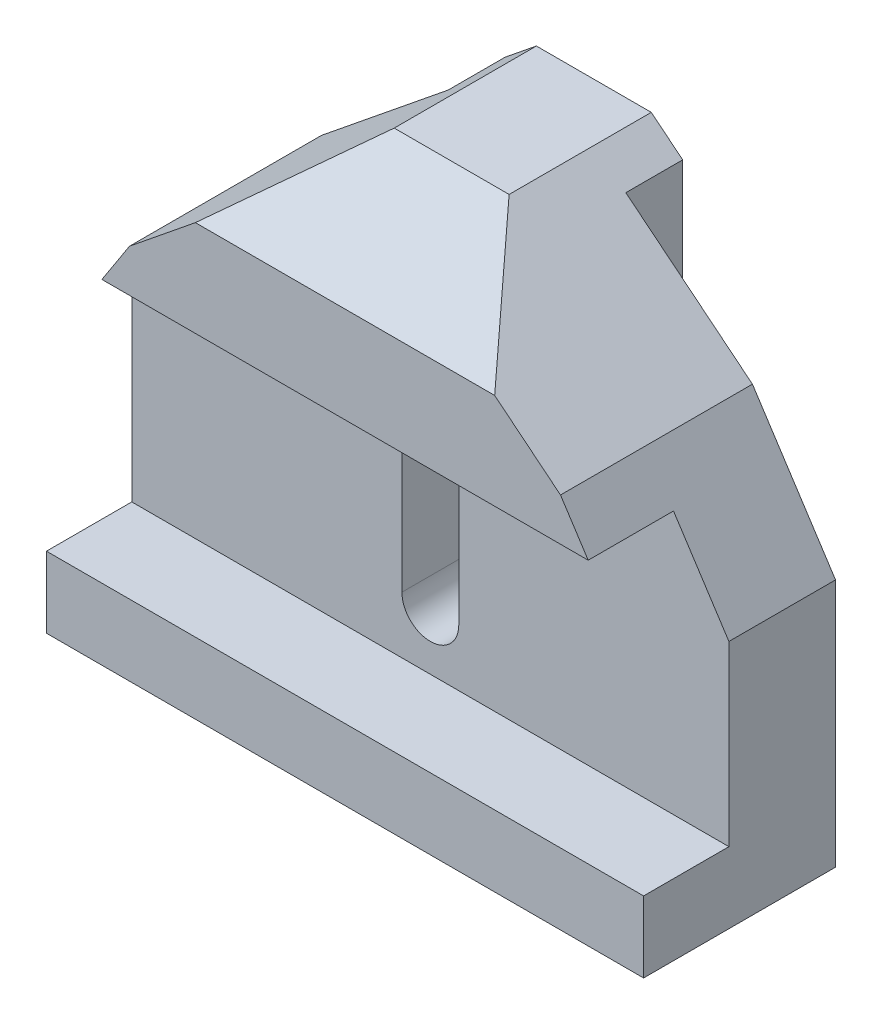
ISO-10303-21;
HEADER;
FILE_DESCRIPTION(('STEP AP214'),'2;1');
FILE_NAME('part.step','',(''),(''),'','','');
FILE_SCHEMA(('AUTOMOTIVE_DESIGN { 1 0 10303 214 1 1 1 1 }'));
ENDSEC;
DATA;
#1=APPLICATION_CONTEXT('core data for automotive mechanical design processes');
#2=APPLICATION_PROTOCOL_DEFINITION('international standard','automotive_design',2000,#1);
#3=PRODUCT_CONTEXT('',#1,'mechanical');
#4=PRODUCT('Part','Part','',(#3));
#5=PRODUCT_RELATED_PRODUCT_CATEGORY('part','',(#4));
#6=PRODUCT_DEFINITION_FORMATION('','',#4);
#7=PRODUCT_DEFINITION_CONTEXT('part definition',#1,'design');
#8=PRODUCT_DEFINITION('design','',#6,#7);
#9=PRODUCT_DEFINITION_SHAPE('','',#8);
#10=(LENGTH_UNIT() NAMED_UNIT(*) SI_UNIT(.MILLI.,.METRE.));
#11=(NAMED_UNIT(*) PLANE_ANGLE_UNIT() SI_UNIT($,.RADIAN.));
#12=(NAMED_UNIT(*) SI_UNIT($,.STERADIAN.) SOLID_ANGLE_UNIT());
#13=UNCERTAINTY_MEASURE_WITH_UNIT(LENGTH_MEASURE(1.E-05),#10,'distance_accuracy_value','');
#14=(GEOMETRIC_REPRESENTATION_CONTEXT(3) GLOBAL_UNCERTAINTY_ASSIGNED_CONTEXT((#13)) GLOBAL_UNIT_ASSIGNED_CONTEXT((#10,
#11,#12)) REPRESENTATION_CONTEXT('',''));
#15=CARTESIAN_POINT('',(0.,0.,0.));
#16=DIRECTION('',(0.,0.,1.));
#17=DIRECTION('',(1.,0.,0.));
#18=AXIS2_PLACEMENT_3D('',#15,#16,#17);
#19=CARTESIAN_POINT('',(-84.,0.,23.));
#20=DIRECTION('',(0.,0.,1.));
#21=DIRECTION('',(0.,-1.,0.));
#22=AXIS2_PLACEMENT_3D('',#19,#20,#21);
#23=PLANE('',#22);
#24=CARTESIAN_POINT('',(-42.,18.,23.));
#25=DIRECTION('',(0.,0.,1.));
#26=DIRECTION('',(1.,0.,0.));
#27=AXIS2_PLACEMENT_3D('',#24,#25,#26);
#28=CIRCLE('',#27,4.);
#29=CARTESIAN_POINT('',(-46.,18.,23.));
#30=VERTEX_POINT('',#29);
#31=CARTESIAN_POINT('',(-38.,18.,23.));
#32=VERTEX_POINT('',#31);
#33=EDGE_CURVE('E54',#30,#32,#28,.T.);
#34=ORIENTED_EDGE('',*,*,#33,.F.);
#35=DIRECTION('',(0.,1.,0.));
#36=VECTOR('',#35,1.);
#37=CARTESIAN_POINT('',(-46.,18.,23.));
#38=LINE('',#37,#36);
#39=CARTESIAN_POINT('',(-46.,39.,23.));
#40=VERTEX_POINT('',#39);
#41=EDGE_CURVE('E199',#30,#40,#38,.T.);
#42=ORIENTED_EDGE('',*,*,#41,.T.);
#43=CARTESIAN_POINT('',(-42.,39.,23.));
#44=DIRECTION('',(0.,0.,1.));
#45=DIRECTION('',(1.,0.,0.));
#46=AXIS2_PLACEMENT_3D('',#43,#44,#45);
#47=CIRCLE('',#46,4.);
#48=CARTESIAN_POINT('',(-38.,39.,23.));
#49=VERTEX_POINT('',#48);
#50=EDGE_CURVE('E184',#49,#40,#47,.T.);
#51=ORIENTED_EDGE('',*,*,#50,.F.);
#52=DIRECTION('',(0.,1.,0.));
#53=VECTOR('',#52,1.);
#54=CARTESIAN_POINT('',(-38.,18.,23.));
#55=LINE('',#54,#53);
#56=EDGE_CURVE('E191',#32,#49,#55,.T.);
#57=ORIENTED_EDGE('',*,*,#56,.F.);
#58=EDGE_LOOP('',(#34,#42,#51,#57));
#59=FACE_BOUND('',#58,.T.);
#60=DIRECTION('',(0.544639035015022,-0.838670567945427,0.));
#61=VECTOR('',#60,1.);
#62=CARTESIAN_POINT('',(-8.93001548207051,48.7510179671623,23.));
#63=LINE('',#62,#61);
#64=CARTESIAN_POINT('',(-7.79289111837003,47.,23.));
#65=VERTEX_POINT('',#64);
#66=CARTESIAN_POINT('',(0.,35.,23.));
#67=VERTEX_POINT('',#66);
#68=EDGE_CURVE('E262',#65,#67,#63,.T.);
#69=ORIENTED_EDGE('',*,*,#68,.F.);
#70=DIRECTION('',(1.,0.,0.));
#71=VECTOR('',#70,1.);
#72=CARTESIAN_POINT('',(-84.,47.,23.));
#73=LINE('',#72,#71);
#74=CARTESIAN_POINT('',(-76.20710888163,47.,23.));
#75=VERTEX_POINT('',#74);
#76=EDGE_CURVE('E295',#75,#65,#73,.T.);
#77=ORIENTED_EDGE('',*,*,#76,.F.);
#78=DIRECTION('',(0.544639035015022,0.838670567945427,0.));
#79=VECTOR('',#78,1.);
#80=CARTESIAN_POINT('',(-99.9870455087454,10.3821087461733,23.));
#81=LINE('',#80,#79);
#82=CARTESIAN_POINT('',(-84.,35.,23.));
#83=VERTEX_POINT('',#82);
#84=EDGE_CURVE('E267',#83,#75,#81,.T.);
#85=ORIENTED_EDGE('',*,*,#84,.F.);
#86=DIRECTION('',(0.,-1.,0.));
#87=VECTOR('',#86,1.);
#88=CARTESIAN_POINT('',(-84.,0.,23.));
#89=LINE('',#88,#87);
#90=CARTESIAN_POINT('',(-84.,10.,23.));
#91=VERTEX_POINT('',#90);
#92=EDGE_CURVE('E273',#83,#91,#89,.T.);
#93=ORIENTED_EDGE('',*,*,#92,.T.);
#94=DIRECTION('',(1.,0.,0.));
#95=VECTOR('',#94,1.);
#96=CARTESIAN_POINT('',(-84.,10.,23.));
#97=LINE('',#96,#95);
#98=CARTESIAN_POINT('',(0.,10.,23.));
#99=VERTEX_POINT('',#98);
#100=EDGE_CURVE('E284',#91,#99,#97,.T.);
#101=ORIENTED_EDGE('',*,*,#100,.T.);
#102=DIRECTION('',(0.,-1.,0.));
#103=VECTOR('',#102,1.);
#104=CARTESIAN_POINT('',(0.,0.,23.));
#105=LINE('',#104,#103);
#106=EDGE_CURVE('E274',#67,#99,#105,.T.);
#107=ORIENTED_EDGE('',*,*,#106,.F.);
#108=EDGE_LOOP('',(#69,#77,#85,#93,#101,#107));
#109=FACE_BOUND('',#108,.T.);
#110=ADVANCED_FACE('F41',(#59,#109),#23,.T.);
#111=CARTESIAN_POINT('',(-84.,47.,0.));
#112=DIRECTION('',(0.,-1.,0.));
#113=DIRECTION('',(0.,0.,-1.));
#114=AXIS2_PLACEMENT_3D('',#111,#112,#113);
#115=PLANE('',#114);
#116=DIRECTION('',(0.,0.,-1.));
#117=VECTOR('',#116,1.);
#118=CARTESIAN_POINT('',(-7.79289111837002,47.,0.));
#119=LINE('',#118,#117);
#120=CARTESIAN_POINT('',(-7.79289111837003,47.,35.));
#121=VERTEX_POINT('',#120);
#122=EDGE_CURVE('E254',#121,#65,#119,.T.);
#123=ORIENTED_EDGE('',*,*,#122,.F.);
#124=DIRECTION('',(1.,0.,0.));
#125=VECTOR('',#124,1.);
#126=CARTESIAN_POINT('',(-84.,47.,35.));
#127=LINE('',#126,#125);
#128=CARTESIAN_POINT('',(-76.20710888163,47.,35.));
#129=VERTEX_POINT('',#128);
#130=EDGE_CURVE('E296',#129,#121,#127,.T.);
#131=ORIENTED_EDGE('',*,*,#130,.F.);
#132=DIRECTION('',(0.,0.,1.));
#133=VECTOR('',#132,1.);
#134=CARTESIAN_POINT('',(-76.20710888163,47.,0.));
#135=LINE('',#134,#133);
#136=EDGE_CURVE('E268',#75,#129,#135,.T.);
#137=ORIENTED_EDGE('',*,*,#136,.F.);
#138=ORIENTED_EDGE('',*,*,#76,.T.);
#139=EDGE_LOOP('',(#123,#131,#137,#138));
#140=FACE_BOUND('',#139,.T.);
#141=ADVANCED_FACE('F368',(#140),#115,.T.);
#142=CARTESIAN_POINT('',(-84.,0.,35.));
#143=DIRECTION('',(0.,0.,1.));
#144=DIRECTION('',(1.,0.,0.));
#145=AXIS2_PLACEMENT_3D('',#142,#143,#144);
#146=PLANE('',#145);
#147=DIRECTION('',(0.544639035015022,-0.838670567945427,0.));
#148=VECTOR('',#147,1.);
#149=CARTESIAN_POINT('',(0.,35.,35.));
#150=LINE('',#149,#148);
#151=CARTESIAN_POINT('',(-11.689336677555,53.,35.));
#152=VERTEX_POINT('',#151);
#153=EDGE_CURVE('E250',#152,#121,#150,.T.);
#154=ORIENTED_EDGE('',*,*,#153,.F.);
#155=DIRECTION('',(0.777145961456972,-0.629320391049836,0.));
#156=VECTOR('',#155,1.);
#157=CARTESIAN_POINT('',(-11.689336677555,53.,35.));
#158=LINE('',#157,#156);
#159=CARTESIAN_POINT('',(-20.9472210263923,60.4968869268543,35.));
#160=VERTEX_POINT('',#159);
#161=EDGE_CURVE('E242',#160,#152,#158,.T.);
#162=ORIENTED_EDGE('',*,*,#161,.F.);
#163=DIRECTION('',(1.,0.,0.));
#164=VECTOR('',#163,1.);
#165=CARTESIAN_POINT('',(-84.,60.4968869268543,35.));
#166=LINE('',#165,#164);
#167=CARTESIAN_POINT('',(-63.0527789736078,60.4968869268543,35.));
#168=VERTEX_POINT('',#167);
#169=EDGE_CURVE('E301',#168,#160,#166,.T.);
#170=ORIENTED_EDGE('',*,*,#169,.F.);
#171=DIRECTION('',(0.777145961456972,0.629320391049836,0.));
#172=VECTOR('',#171,1.);
#173=CARTESIAN_POINT('',(-72.310663322445,53.,35.));
#174=LINE('',#173,#172);
#175=CARTESIAN_POINT('',(-72.310663322445,53.,35.));
#176=VERTEX_POINT('',#175);
#177=EDGE_CURVE('E260',#176,#168,#174,.T.);
#178=ORIENTED_EDGE('',*,*,#177,.F.);
#179=DIRECTION('',(0.544639035015022,0.838670567945427,0.));
#180=VECTOR('',#179,1.);
#181=CARTESIAN_POINT('',(-84.,35.,35.));
#182=LINE('',#181,#180);
#183=EDGE_CURVE('E247',#129,#176,#182,.T.);
#184=ORIENTED_EDGE('',*,*,#183,.F.);
#185=ORIENTED_EDGE('',*,*,#130,.T.);
#186=EDGE_LOOP('',(#154,#162,#170,#178,#184,#185));
#187=FACE_BOUND('',#186,.T.);
#188=ADVANCED_FACE('F375',(#187),#146,.T.);
#189=CARTESIAN_POINT('',(-84.,57.0386412959202,39.9388866046431));
#190=DIRECTION('',(0.,0.819152044288991,0.573576436351047));
#191=DIRECTION('',(0.,-0.573576436351047,0.819152044288991));
#192=AXIS2_PLACEMENT_3D('',#189,#190,#191);
#193=PLANE('',#192);
#194=DIRECTION('',(0.578003525978811,-0.468058026468054,0.668456137539998));
#195=VECTOR('',#194,1.);
#196=CARTESIAN_POINT('',(-39.1685740328013,75.2522476546541,13.9271609878319));
#197=LINE('',#196,#195);
#198=CARTESIAN_POINT('',(-33.9174854951861,71.,20.));
#199=VERTEX_POINT('',#198);
#200=EDGE_CURVE('E275',#199,#160,#197,.T.);
#201=ORIENTED_EDGE('',*,*,#200,.F.);
#202=DIRECTION('',(1.,0.,0.));
#203=VECTOR('',#202,1.);
#204=CARTESIAN_POINT('',(-84.,71.,20.));
#205=LINE('',#204,#203);
#206=CARTESIAN_POINT('',(-50.082514504814,71.,20.));
#207=VERTEX_POINT('',#206);
#208=EDGE_CURVE('E302',#207,#199,#205,.T.);
#209=ORIENTED_EDGE('',*,*,#208,.F.);
#210=DIRECTION('',(0.578003525978811,0.468058026468054,-0.668456137539998));
#211=VECTOR('',#210,1.);
#212=CARTESIAN_POINT('',(-72.8948243548895,52.5269557231117,46.3822413624967));
#213=LINE('',#212,#211);
#214=EDGE_CURVE('E266',#168,#207,#213,.T.);
#215=ORIENTED_EDGE('',*,*,#214,.F.);
#216=ORIENTED_EDGE('',*,*,#169,.T.);
#217=EDGE_LOOP('',(#201,#209,#215,#216));
#218=FACE_BOUND('',#217,.T.);
#219=ADVANCED_FACE('F378',(#218),#193,.T.);
#220=CARTESIAN_POINT('',(-84.,71.,0.));
#221=DIRECTION('',(0.,1.,0.));
#222=DIRECTION('',(0.,0.,1.));
#223=AXIS2_PLACEMENT_3D('',#220,#221,#222);
#224=PLANE('',#223);
#225=DIRECTION('',(0.,0.,1.));
#226=VECTOR('',#225,1.);
#227=CARTESIAN_POINT('',(-33.9174854951861,71.,-49.));
#228=LINE('',#227,#226);
#229=CARTESIAN_POINT('',(-33.9174854951861,71.,0.));
#230=VERTEX_POINT('',#229);
#231=EDGE_CURVE('E249',#230,#199,#228,.T.);
#232=ORIENTED_EDGE('',*,*,#231,.F.);
#233=DIRECTION('',(1.,0.,0.));
#234=VECTOR('',#233,1.);
#235=CARTESIAN_POINT('',(-84.,71.,0.));
#236=LINE('',#235,#234);
#237=CARTESIAN_POINT('',(-50.082514504814,71.,0.));
#238=VERTEX_POINT('',#237);
#239=EDGE_CURVE('E310',#238,#230,#236,.T.);
#240=ORIENTED_EDGE('',*,*,#239,.F.);
#241=DIRECTION('',(0.,0.,1.));
#242=VECTOR('',#241,1.);
#243=CARTESIAN_POINT('',(-50.082514504814,71.,-49.));
#244=LINE('',#243,#242);
#245=EDGE_CURVE('E243',#238,#207,#244,.T.);
#246=ORIENTED_EDGE('',*,*,#245,.T.);
#247=ORIENTED_EDGE('',*,*,#208,.T.);
#248=EDGE_LOOP('',(#232,#240,#246,#247));
#249=FACE_BOUND('',#248,.T.);
#250=ADVANCED_FACE('F386',(#249),#224,.T.);
#251=CARTESIAN_POINT('',(-84.,0.,0.));
#252=DIRECTION('',(0.,0.,-1.));
#253=DIRECTION('',(-1.,0.,0.));
#254=AXIS2_PLACEMENT_3D('',#251,#252,#253);
#255=PLANE('',#254);
#256=CARTESIAN_POINT('',(-42.,18.,0.));
#257=DIRECTION('',(0.,0.,-1.));
#258=DIRECTION('',(-1.,0.,0.));
#259=AXIS2_PLACEMENT_3D('',#256,#257,#258);
#260=CIRCLE('',#259,4.);
#261=CARTESIAN_POINT('',(-38.,18.,0.));
#262=VERTEX_POINT('',#261);
#263=CARTESIAN_POINT('',(-46.,18.,0.));
#264=VERTEX_POINT('',#263);
#265=EDGE_CURVE('E11',#262,#264,#260,.T.);
#266=ORIENTED_EDGE('',*,*,#265,.F.);
#267=DIRECTION('',(0.,-1.,0.));
#268=VECTOR('',#267,1.);
#269=CARTESIAN_POINT('',(-38.,0.,0.));
#270=LINE('',#269,#268);
#271=CARTESIAN_POINT('',(-38.,39.,0.));
#272=VERTEX_POINT('',#271);
#273=EDGE_CURVE('E345',#272,#262,#270,.T.);
#274=ORIENTED_EDGE('',*,*,#273,.F.);
#275=CARTESIAN_POINT('',(-42.,39.,0.));
#276=DIRECTION('',(0.,0.,-1.));
#277=DIRECTION('',(-1.,0.,0.));
#278=AXIS2_PLACEMENT_3D('',#275,#276,#277);
#279=CIRCLE('',#278,4.);
#280=CARTESIAN_POINT('',(-46.,39.,0.));
#281=VERTEX_POINT('',#280);
#282=EDGE_CURVE('E189',#281,#272,#279,.T.);
#283=ORIENTED_EDGE('',*,*,#282,.F.);
#284=DIRECTION('',(0.,-1.,0.));
#285=VECTOR('',#284,1.);
#286=CARTESIAN_POINT('',(-46.,0.,0.));
#287=LINE('',#286,#285);
#288=EDGE_CURVE('E48',#281,#264,#287,.T.);
#289=ORIENTED_EDGE('',*,*,#288,.T.);
#290=EDGE_LOOP('',(#266,#274,#283,#289));
#291=FACE_BOUND('',#290,.T.);
#292=DIRECTION('',(0.,1.,0.));
#293=VECTOR('',#292,1.);
#294=CARTESIAN_POINT('',(-54.5,-33.,0.));
#295=LINE('',#294,#293);
#296=CARTESIAN_POINT('',(-54.5,0.,0.));
#297=VERTEX_POINT('',#296);
#298=CARTESIAN_POINT('',(-54.5,67.4227907791278,0.));
#299=VERTEX_POINT('',#298);
#300=EDGE_CURVE('E208',#297,#299,#295,.T.);
#301=ORIENTED_EDGE('',*,*,#300,.T.);
#302=DIRECTION('',(-0.777145961456972,-0.629320391049836,0.));
#303=VECTOR('',#302,1.);
#304=CARTESIAN_POINT('',(-105.291417957253,26.2927114940107,0.));
#305=LINE('',#304,#303);
#306=EDGE_CURVE('E323',#238,#299,#305,.T.);
#307=ORIENTED_EDGE('',*,*,#306,.F.);
#308=ORIENTED_EDGE('',*,*,#239,.T.);
#309=DIRECTION('',(-0.777145961456972,0.629320391049836,0.));
#310=VECTOR('',#309,1.);
#311=CARTESIAN_POINT('',(-29.4408730570935,67.3749107248305,0.));
#312=LINE('',#311,#310);
#313=CARTESIAN_POINT('',(-29.5,67.4227907791278,0.));
#314=VERTEX_POINT('',#313);
#315=EDGE_CURVE('E328',#314,#230,#312,.T.);
#316=ORIENTED_EDGE('',*,*,#315,.F.);
#317=DIRECTION('',(0.,1.,0.));
#318=VECTOR('',#317,1.);
#319=CARTESIAN_POINT('',(-29.5,-33.,0.));
#320=LINE('',#319,#318);
#321=CARTESIAN_POINT('',(-29.5,0.,0.));
#322=VERTEX_POINT('',#321);
#323=EDGE_CURVE('E217',#322,#314,#320,.T.);
#324=ORIENTED_EDGE('',*,*,#323,.F.);
#325=DIRECTION('',(1.,0.,0.));
#326=VECTOR('',#325,1.);
#327=CARTESIAN_POINT('',(-84.,0.,0.));
#328=LINE('',#327,#326);
#329=EDGE_CURVE('E309',#297,#322,#328,.T.);
#330=ORIENTED_EDGE('',*,*,#329,.F.);
#331=EDGE_LOOP('',(#301,#307,#308,#316,#324,#330));
#332=FACE_BOUND('',#331,.T.);
#333=ADVANCED_FACE('F350',(#291,#332),#255,.T.);
#334=CARTESIAN_POINT('',(-84.,0.,0.));
#335=DIRECTION('',(0.,1.,0.));
#336=DIRECTION('',(0.,0.,1.));
#337=AXIS2_PLACEMENT_3D('',#334,#335,#336);
#338=PLANE('',#337);
#339=DIRECTION('',(1.,0.,0.));
#340=VECTOR('',#339,1.);
#341=CARTESIAN_POINT('',(-84.,0.,8.));
#342=LINE('',#341,#340);
#343=CARTESIAN_POINT('',(-84.,0.,8.));
#344=VERTEX_POINT('',#343);
#345=CARTESIAN_POINT('',(-54.5,0.,8.));
#346=VERTEX_POINT('',#345);
#347=EDGE_CURVE('E226',#344,#346,#342,.T.);
#348=ORIENTED_EDGE('',*,*,#347,.T.);
#349=DIRECTION('',(0.,0.,-1.));
#350=VECTOR('',#349,1.);
#351=CARTESIAN_POINT('',(-54.5,0.,0.));
#352=LINE('',#351,#350);
#353=EDGE_CURVE('E233',#346,#297,#352,.T.);
#354=ORIENTED_EDGE('',*,*,#353,.T.);
#355=ORIENTED_EDGE('',*,*,#329,.T.);
#356=DIRECTION('',(0.,0.,1.));
#357=VECTOR('',#356,1.);
#358=CARTESIAN_POINT('',(-29.5,0.,0.));
#359=LINE('',#358,#357);
#360=CARTESIAN_POINT('',(-29.5,0.,7.99999999999999));
#361=VERTEX_POINT('',#360);
#362=EDGE_CURVE('E234',#322,#361,#359,.T.);
#363=ORIENTED_EDGE('',*,*,#362,.T.);
#364=DIRECTION('',(1.,0.,0.));
#365=VECTOR('',#364,1.);
#366=CARTESIAN_POINT('',(-84.,0.,7.99999999999998));
#367=LINE('',#366,#365);
#368=CARTESIAN_POINT('',(0.,0.,7.99999999999999));
#369=VERTEX_POINT('',#368);
#370=EDGE_CURVE('E239',#361,#369,#367,.T.);
#371=ORIENTED_EDGE('',*,*,#370,.T.);
#372=DIRECTION('',(0.,0.,1.));
#373=VECTOR('',#372,1.);
#374=CARTESIAN_POINT('',(0.,0.,0.));
#375=LINE('',#374,#373);
#376=CARTESIAN_POINT('',(0.,0.,35.));
#377=VERTEX_POINT('',#376);
#378=EDGE_CURVE('E279',#369,#377,#375,.T.);
#379=ORIENTED_EDGE('',*,*,#378,.T.);
#380=DIRECTION('',(1.,0.,0.));
#381=VECTOR('',#380,1.);
#382=CARTESIAN_POINT('',(-84.,0.,35.));
#383=LINE('',#382,#381);
#384=CARTESIAN_POINT('',(-84.,0.,35.));
#385=VERTEX_POINT('',#384);
#386=EDGE_CURVE('E312',#385,#377,#383,.T.);
#387=ORIENTED_EDGE('',*,*,#386,.F.);
#388=DIRECTION('',(0.,0.,1.));
#389=VECTOR('',#388,1.);
#390=CARTESIAN_POINT('',(-84.,0.,0.));
#391=LINE('',#390,#389);
#392=EDGE_CURVE('E283',#344,#385,#391,.T.);
#393=ORIENTED_EDGE('',*,*,#392,.F.);
#394=EDGE_LOOP('',(#348,#354,#355,#363,#371,#379,#387,#393));
#395=FACE_BOUND('',#394,.T.);
#396=ADVANCED_FACE('F394',(#395),#338,.F.);
#397=CARTESIAN_POINT('',(-84.,0.,35.));
#398=DIRECTION('',(0.,0.,-1.));
#399=DIRECTION('',(-1.,0.,0.));
#400=AXIS2_PLACEMENT_3D('',#397,#398,#399);
#401=PLANE('',#400);
#402=DIRECTION('',(0.,1.,0.));
#403=VECTOR('',#402,1.);
#404=CARTESIAN_POINT('',(0.,0.,35.));
#405=LINE('',#404,#403);
#406=CARTESIAN_POINT('',(0.,10.,35.));
#407=VERTEX_POINT('',#406);
#408=EDGE_CURVE('E286',#377,#407,#405,.T.);
#409=ORIENTED_EDGE('',*,*,#408,.T.);
#410=DIRECTION('',(1.,0.,0.));
#411=VECTOR('',#410,1.);
#412=CARTESIAN_POINT('',(-84.,10.,35.));
#413=LINE('',#412,#411);
#414=CARTESIAN_POINT('',(-84.,10.,35.));
#415=VERTEX_POINT('',#414);
#416=EDGE_CURVE('E317',#415,#407,#413,.T.);
#417=ORIENTED_EDGE('',*,*,#416,.F.);
#418=DIRECTION('',(0.,1.,0.));
#419=VECTOR('',#418,1.);
#420=CARTESIAN_POINT('',(-84.,0.,35.));
#421=LINE('',#420,#419);
#422=EDGE_CURVE('E281',#385,#415,#421,.T.);
#423=ORIENTED_EDGE('',*,*,#422,.F.);
#424=ORIENTED_EDGE('',*,*,#386,.T.);
#425=EDGE_LOOP('',(#409,#417,#423,#424));
#426=FACE_BOUND('',#425,.T.);
#427=ADVANCED_FACE('F397',(#426),#401,.F.);
#428=CARTESIAN_POINT('',(-84.,10.,0.));
#429=DIRECTION('',(0.,1.,0.));
#430=DIRECTION('',(0.,0.,1.));
#431=AXIS2_PLACEMENT_3D('',#428,#429,#430);
#432=PLANE('',#431);
#433=DIRECTION('',(0.,0.,1.));
#434=VECTOR('',#433,1.);
#435=CARTESIAN_POINT('',(0.,10.,0.));
#436=LINE('',#435,#434);
#437=EDGE_CURVE('E289',#99,#407,#436,.T.);
#438=ORIENTED_EDGE('',*,*,#437,.F.);
#439=ORIENTED_EDGE('',*,*,#100,.F.);
#440=DIRECTION('',(0.,0.,1.));
#441=VECTOR('',#440,1.);
#442=CARTESIAN_POINT('',(-84.,10.,0.));
#443=LINE('',#442,#441);
#444=EDGE_CURVE('E280',#91,#415,#443,.T.);
#445=ORIENTED_EDGE('',*,*,#444,.T.);
#446=ORIENTED_EDGE('',*,*,#416,.T.);
#447=EDGE_LOOP('',(#438,#439,#445,#446));
#448=FACE_BOUND('',#447,.T.);
#449=ADVANCED_FACE('F402',(#448),#432,.T.);
#450=CARTESIAN_POINT('',(-84.,0.,0.));
#451=DIRECTION('',(1.,0.,0.));
#452=DIRECTION('',(0.,0.,-1.));
#453=AXIS2_PLACEMENT_3D('',#450,#451,#452);
#454=PLANE('',#453);
#455=DIRECTION('',(0.,0.,-1.));
#456=VECTOR('',#455,1.);
#457=CARTESIAN_POINT('',(-84.,35.,0.));
#458=LINE('',#457,#456);
#459=CARTESIAN_POINT('',(-84.,35.,8.00000000000001));
#460=VERTEX_POINT('',#459);
#461=EDGE_CURVE('E325',#83,#460,#458,.T.);
#462=ORIENTED_EDGE('',*,*,#461,.T.);
#463=DIRECTION('',(0.,1.,0.));
#464=VECTOR('',#463,1.);
#465=CARTESIAN_POINT('',(-84.,-33.,8.));
#466=LINE('',#465,#464);
#467=EDGE_CURVE('E220',#344,#460,#466,.T.);
#468=ORIENTED_EDGE('',*,*,#467,.F.);
#469=ORIENTED_EDGE('',*,*,#392,.T.);
#470=ORIENTED_EDGE('',*,*,#422,.T.);
#471=ORIENTED_EDGE('',*,*,#444,.F.);
#472=ORIENTED_EDGE('',*,*,#92,.F.);
#473=EDGE_LOOP('',(#462,#468,#469,#470,#471,#472));
#474=FACE_BOUND('',#473,.T.);
#475=ADVANCED_FACE('F401',(#474),#454,.F.);
#476=CARTESIAN_POINT('',(0.,0.,0.));
#477=DIRECTION('',(1.,0.,0.));
#478=DIRECTION('',(0.,0.,-1.));
#479=AXIS2_PLACEMENT_3D('',#476,#477,#478);
#480=PLANE('',#479);
#481=DIRECTION('',(0.,1.,0.));
#482=VECTOR('',#481,1.);
#483=CARTESIAN_POINT('',(0.,-33.,7.99999999999999));
#484=LINE('',#483,#482);
#485=CARTESIAN_POINT('',(0.,35.,7.99999999999999));
#486=VERTEX_POINT('',#485);
#487=EDGE_CURVE('E210',#369,#486,#484,.T.);
#488=ORIENTED_EDGE('',*,*,#487,.T.);
#489=DIRECTION('',(0.,0.,-1.));
#490=VECTOR('',#489,1.);
#491=CARTESIAN_POINT('',(0.,35.,0.));
#492=LINE('',#491,#490);
#493=EDGE_CURVE('E300',#67,#486,#492,.T.);
#494=ORIENTED_EDGE('',*,*,#493,.F.);
#495=ORIENTED_EDGE('',*,*,#106,.T.);
#496=ORIENTED_EDGE('',*,*,#437,.T.);
#497=ORIENTED_EDGE('',*,*,#408,.F.);
#498=ORIENTED_EDGE('',*,*,#378,.F.);
#499=EDGE_LOOP('',(#488,#494,#495,#496,#497,#498));
#500=FACE_BOUND('',#499,.T.);
#501=ADVANCED_FACE('F381',(#500),#480,.T.);
#502=CARTESIAN_POINT('',(0.,35.,-49.));
#503=DIRECTION('',(-0.838670567945427,-0.544639035015022,0.));
#504=DIRECTION('',(0.544639035015022,-0.838670567945427,0.));
#505=AXIS2_PLACEMENT_3D('',#502,#503,#504);
#506=PLANE('',#505);
#507=ORIENTED_EDGE('',*,*,#493,.T.);
#508=DIRECTION('',(-0.544639035015022,0.838670567945427,0.));
#509=VECTOR('',#508,1.);
#510=CARTESIAN_POINT('',(0.,35.,7.99999999999999));
#511=LINE('',#510,#509);
#512=CARTESIAN_POINT('',(-11.689336677555,53.,7.99999999999999));
#513=VERTEX_POINT('',#512);
#514=EDGE_CURVE('E240',#486,#513,#511,.T.);
#515=ORIENTED_EDGE('',*,*,#514,.T.);
#516=DIRECTION('',(0.,0.,1.));
#517=VECTOR('',#516,1.);
#518=CARTESIAN_POINT('',(-11.689336677555,53.,-49.));
#519=LINE('',#518,#517);
#520=EDGE_CURVE('E252',#513,#152,#519,.T.);
#521=ORIENTED_EDGE('',*,*,#520,.T.);
#522=ORIENTED_EDGE('',*,*,#153,.T.);
#523=ORIENTED_EDGE('',*,*,#122,.T.);
#524=ORIENTED_EDGE('',*,*,#68,.T.);
#525=EDGE_LOOP('',(#507,#515,#521,#522,#523,#524));
#526=FACE_BOUND('',#525,.T.);
#527=ADVANCED_FACE('F426',(#526),#506,.F.);
#528=CARTESIAN_POINT('',(-11.689336677555,53.,-49.));
#529=DIRECTION('',(-0.629320391049836,-0.777145961456972,0.));
#530=DIRECTION('',(0.777145961456973,-0.629320391049836,0.));
#531=AXIS2_PLACEMENT_3D('',#528,#529,#530);
#532=PLANE('',#531);
#533=ORIENTED_EDGE('',*,*,#520,.F.);
#534=DIRECTION('',(-0.777145961456972,0.629320391049836,0.));
#535=VECTOR('',#534,1.);
#536=CARTESIAN_POINT('',(-11.689336677555,53.,7.99999999999999));
#537=LINE('',#536,#535);
#538=CARTESIAN_POINT('',(-29.5,67.4227907791278,7.99999999999999));
#539=VERTEX_POINT('',#538);
#540=EDGE_CURVE('E339',#513,#539,#537,.T.);
#541=ORIENTED_EDGE('',*,*,#540,.T.);
#542=DIRECTION('',(0.,0.,-1.));
#543=VECTOR('',#542,1.);
#544=CARTESIAN_POINT('',(-29.5,67.4227907791278,-49.));
#545=LINE('',#544,#543);
#546=EDGE_CURVE('E337',#539,#314,#545,.T.);
#547=ORIENTED_EDGE('',*,*,#546,.T.);
#548=ORIENTED_EDGE('',*,*,#315,.T.);
#549=ORIENTED_EDGE('',*,*,#231,.T.);
#550=ORIENTED_EDGE('',*,*,#200,.T.);
#551=ORIENTED_EDGE('',*,*,#161,.T.);
#552=EDGE_LOOP('',(#533,#541,#547,#548,#549,#550,#551));
#553=FACE_BOUND('',#552,.T.);
#554=ADVANCED_FACE('F467',(#553),#532,.F.);
#555=CARTESIAN_POINT('',(-72.310663322445,53.,-49.));
#556=DIRECTION('',(0.629320391049836,-0.777145961456972,0.));
#557=DIRECTION('',(0.777145961456973,0.629320391049836,0.));
#558=AXIS2_PLACEMENT_3D('',#555,#556,#557);
#559=PLANE('',#558);
#560=ORIENTED_EDGE('',*,*,#306,.T.);
#561=DIRECTION('',(0.,0.,1.));
#562=VECTOR('',#561,1.);
#563=CARTESIAN_POINT('',(-54.5,67.4227907791278,-49.));
#564=LINE('',#563,#562);
#565=CARTESIAN_POINT('',(-54.5,67.4227907791278,8.));
#566=VERTEX_POINT('',#565);
#567=EDGE_CURVE('E332',#299,#566,#564,.T.);
#568=ORIENTED_EDGE('',*,*,#567,.T.);
#569=DIRECTION('',(-0.777145961456972,-0.629320391049836,0.));
#570=VECTOR('',#569,1.);
#571=CARTESIAN_POINT('',(-72.310663322445,53.,8.));
#572=LINE('',#571,#570);
#573=CARTESIAN_POINT('',(-72.310663322445,53.,8.00000000000001));
#574=VERTEX_POINT('',#573);
#575=EDGE_CURVE('E214',#566,#574,#572,.T.);
#576=ORIENTED_EDGE('',*,*,#575,.T.);
#577=DIRECTION('',(0.,0.,1.));
#578=VECTOR('',#577,1.);
#579=CARTESIAN_POINT('',(-72.310663322445,53.,-49.));
#580=LINE('',#579,#578);
#581=EDGE_CURVE('E253',#574,#176,#580,.T.);
#582=ORIENTED_EDGE('',*,*,#581,.T.);
#583=ORIENTED_EDGE('',*,*,#177,.T.);
#584=ORIENTED_EDGE('',*,*,#214,.T.);
#585=ORIENTED_EDGE('',*,*,#245,.F.);
#586=EDGE_LOOP('',(#560,#568,#576,#582,#583,#584,#585));
#587=FACE_BOUND('',#586,.T.);
#588=ADVANCED_FACE('F445',(#587),#559,.F.);
#589=CARTESIAN_POINT('',(-84.,35.,-49.));
#590=DIRECTION('',(0.838670567945427,-0.544639035015022,0.));
#591=DIRECTION('',(0.544639035015022,0.838670567945427,0.));
#592=AXIS2_PLACEMENT_3D('',#589,#590,#591);
#593=PLANE('',#592);
#594=ORIENTED_EDGE('',*,*,#581,.F.);
#595=DIRECTION('',(-0.544639035015022,-0.838670567945427,0.));
#596=VECTOR('',#595,1.);
#597=CARTESIAN_POINT('',(-84.,35.,8.00000000000001));
#598=LINE('',#597,#596);
#599=EDGE_CURVE('E329',#574,#460,#598,.T.);
#600=ORIENTED_EDGE('',*,*,#599,.T.);
#601=ORIENTED_EDGE('',*,*,#461,.F.);
#602=ORIENTED_EDGE('',*,*,#84,.T.);
#603=ORIENTED_EDGE('',*,*,#136,.T.);
#604=ORIENTED_EDGE('',*,*,#183,.T.);
#605=EDGE_LOOP('',(#594,#600,#601,#602,#603,#604));
#606=FACE_BOUND('',#605,.T.);
#607=ADVANCED_FACE('F434',(#606),#593,.F.);
#608=CARTESIAN_POINT('',(-54.5,-33.,0.));
#609=DIRECTION('',(1.,0.,0.));
#610=DIRECTION('',(0.,0.,-1.));
#611=AXIS2_PLACEMENT_3D('',#608,#609,#610);
#612=PLANE('',#611);
#613=DIRECTION('',(0.,1.,0.));
#614=VECTOR('',#613,1.);
#615=CARTESIAN_POINT('',(-54.5,-33.,8.));
#616=LINE('',#615,#614);
#617=EDGE_CURVE('E211',#346,#566,#616,.T.);
#618=ORIENTED_EDGE('',*,*,#617,.T.);
#619=ORIENTED_EDGE('',*,*,#567,.F.);
#620=ORIENTED_EDGE('',*,*,#300,.F.);
#621=ORIENTED_EDGE('',*,*,#353,.F.);
#622=EDGE_LOOP('',(#618,#619,#620,#621));
#623=FACE_BOUND('',#622,.T.);
#624=ADVANCED_FACE('F455',(#623),#612,.F.);
#625=CARTESIAN_POINT('',(-84.,-33.,8.));
#626=DIRECTION('',(0.,0.,1.));
#627=DIRECTION('',(1.,0.,0.));
#628=AXIS2_PLACEMENT_3D('',#625,#626,#627);
#629=PLANE('',#628);
#630=ORIENTED_EDGE('',*,*,#467,.T.);
#631=ORIENTED_EDGE('',*,*,#599,.F.);
#632=ORIENTED_EDGE('',*,*,#575,.F.);
#633=ORIENTED_EDGE('',*,*,#617,.F.);
#634=ORIENTED_EDGE('',*,*,#347,.F.);
#635=EDGE_LOOP('',(#630,#631,#632,#633,#634));
#636=FACE_BOUND('',#635,.T.);
#637=ADVANCED_FACE('F453',(#636),#629,.F.);
#638=CARTESIAN_POINT('',(0.,-33.,7.99999999999999));
#639=DIRECTION('',(0.,0.,1.));
#640=DIRECTION('',(1.,0.,0.));
#641=AXIS2_PLACEMENT_3D('',#638,#639,#640);
#642=PLANE('',#641);
#643=DIRECTION('',(0.,1.,0.));
#644=VECTOR('',#643,1.);
#645=CARTESIAN_POINT('',(-29.5,-33.,7.99999999999999));
#646=LINE('',#645,#644);
#647=EDGE_CURVE('E223',#361,#539,#646,.T.);
#648=ORIENTED_EDGE('',*,*,#647,.T.);
#649=ORIENTED_EDGE('',*,*,#540,.F.);
#650=ORIENTED_EDGE('',*,*,#514,.F.);
#651=ORIENTED_EDGE('',*,*,#487,.F.);
#652=ORIENTED_EDGE('',*,*,#370,.F.);
#653=EDGE_LOOP('',(#648,#649,#650,#651,#652));
#654=FACE_BOUND('',#653,.T.);
#655=ADVANCED_FACE('F365',(#654),#642,.F.);
#656=CARTESIAN_POINT('',(-29.5,-33.,0.));
#657=DIRECTION('',(-1.,0.,0.));
#658=DIRECTION('',(0.,0.,1.));
#659=AXIS2_PLACEMENT_3D('',#656,#657,#658);
#660=PLANE('',#659);
#661=ORIENTED_EDGE('',*,*,#323,.T.);
#662=ORIENTED_EDGE('',*,*,#546,.F.);
#663=ORIENTED_EDGE('',*,*,#647,.F.);
#664=ORIENTED_EDGE('',*,*,#362,.F.);
#665=EDGE_LOOP('',(#661,#662,#663,#664));
#666=FACE_BOUND('',#665,.T.);
#667=ADVANCED_FACE('F355',(#666),#660,.F.);
#668=CARTESIAN_POINT('',(-42.,18.,-81.));
#669=DIRECTION('',(0.,0.,1.));
#670=DIRECTION('',(1.,0.,0.));
#671=AXIS2_PLACEMENT_3D('',#668,#669,#670);
#672=CYLINDRICAL_SURFACE('',#671,4.);
#673=ORIENTED_EDGE('',*,*,#265,.T.);
#674=DIRECTION('',(0.,0.,1.));
#675=VECTOR('',#674,1.);
#676=CARTESIAN_POINT('',(-46.,18.,-81.));
#677=LINE('',#676,#675);
#678=EDGE_CURVE('E201',#264,#30,#677,.T.);
#679=ORIENTED_EDGE('',*,*,#678,.T.);
#680=ORIENTED_EDGE('',*,*,#33,.T.);
#681=DIRECTION('',(0.,0.,1.));
#682=VECTOR('',#681,1.);
#683=CARTESIAN_POINT('',(-38.,18.,-81.));
#684=LINE('',#683,#682);
#685=EDGE_CURVE('E192',#262,#32,#684,.T.);
#686=ORIENTED_EDGE('',*,*,#685,.F.);
#687=EDGE_LOOP('',(#673,#679,#680,#686));
#688=FACE_BOUND('',#687,.T.);
#689=ADVANCED_FACE('F354',(#688),#672,.F.);
#690=CARTESIAN_POINT('',(-46.,18.,-81.));
#691=DIRECTION('',(1.,0.,0.));
#692=DIRECTION('',(0.,0.,-1.));
#693=AXIS2_PLACEMENT_3D('',#690,#691,#692);
#694=PLANE('',#693);
#695=DIRECTION('',(0.,0.,1.));
#696=VECTOR('',#695,1.);
#697=CARTESIAN_POINT('',(-46.,39.,-81.));
#698=LINE('',#697,#696);
#699=EDGE_CURVE('E188',#281,#40,#698,.T.);
#700=ORIENTED_EDGE('',*,*,#699,.T.);
#701=ORIENTED_EDGE('',*,*,#41,.F.);
#702=ORIENTED_EDGE('',*,*,#678,.F.);
#703=ORIENTED_EDGE('',*,*,#288,.F.);
#704=EDGE_LOOP('',(#700,#701,#702,#703));
#705=FACE_BOUND('',#704,.T.);
#706=ADVANCED_FACE('F353',(#705),#694,.T.);
#707=CARTESIAN_POINT('',(-42.,39.,-81.));
#708=DIRECTION('',(0.,0.,1.));
#709=DIRECTION('',(1.,0.,0.));
#710=AXIS2_PLACEMENT_3D('',#707,#708,#709);
#711=CYLINDRICAL_SURFACE('',#710,4.);
#712=ORIENTED_EDGE('',*,*,#282,.T.);
#713=DIRECTION('',(0.,0.,1.));
#714=VECTOR('',#713,1.);
#715=CARTESIAN_POINT('',(-38.,39.,-81.));
#716=LINE('',#715,#714);
#717=EDGE_CURVE('E64',#272,#49,#716,.T.);
#718=ORIENTED_EDGE('',*,*,#717,.T.);
#719=ORIENTED_EDGE('',*,*,#50,.T.);
#720=ORIENTED_EDGE('',*,*,#699,.F.);
#721=EDGE_LOOP('',(#712,#718,#719,#720));
#722=FACE_BOUND('',#721,.T.);
#723=ADVANCED_FACE('F185',(#722),#711,.F.);
#724=CARTESIAN_POINT('',(-38.,18.,-81.));
#725=DIRECTION('',(1.,0.,0.));
#726=DIRECTION('',(0.,0.,-1.));
#727=AXIS2_PLACEMENT_3D('',#724,#725,#726);
#728=PLANE('',#727);
#729=ORIENTED_EDGE('',*,*,#273,.T.);
#730=ORIENTED_EDGE('',*,*,#685,.T.);
#731=ORIENTED_EDGE('',*,*,#56,.T.);
#732=ORIENTED_EDGE('',*,*,#717,.F.);
#733=EDGE_LOOP('',(#729,#730,#731,#732));
#734=FACE_BOUND('',#733,.T.);
#735=ADVANCED_FACE('F193',(#734),#728,.F.);
#736=CLOSED_SHELL('',(#110,#141,#188,#219,#250,#333,#396,#427,#449,#475,#501,#527,#554,#588,
#607,#624,#637,#655,#667,#689,#706,#723,#735));
#737=MANIFOLD_SOLID_BREP('B2',#736);
#738=ADVANCED_BREP_SHAPE_REPRESENTATION('',(#18,#737),#14);
#739=SHAPE_DEFINITION_REPRESENTATION(#9,#738);
ENDSEC;
END-ISO-10303-21;
